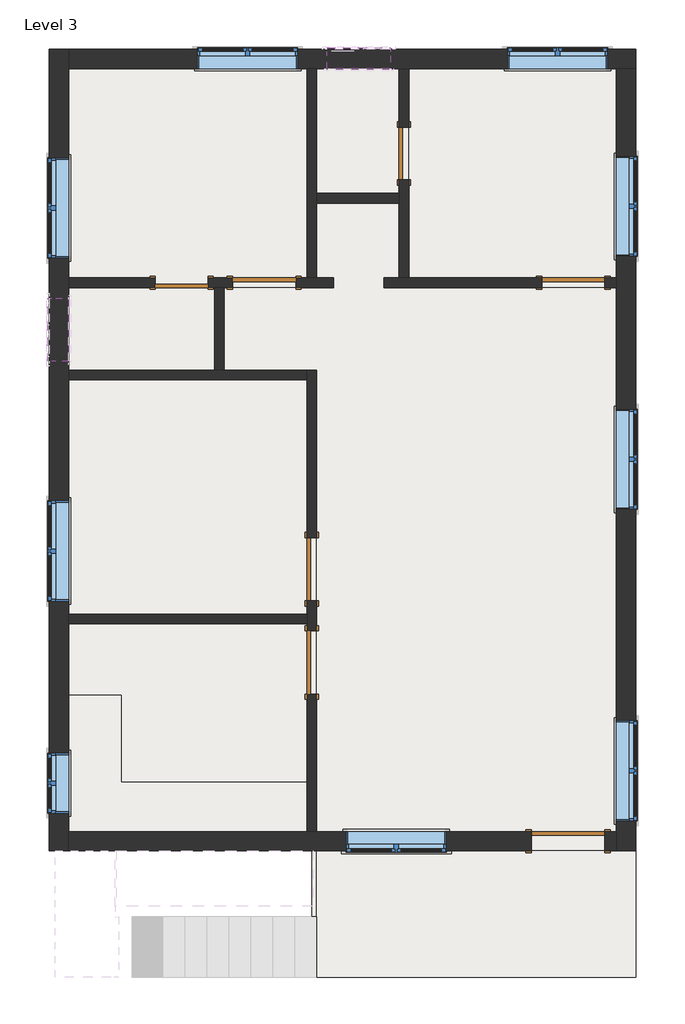
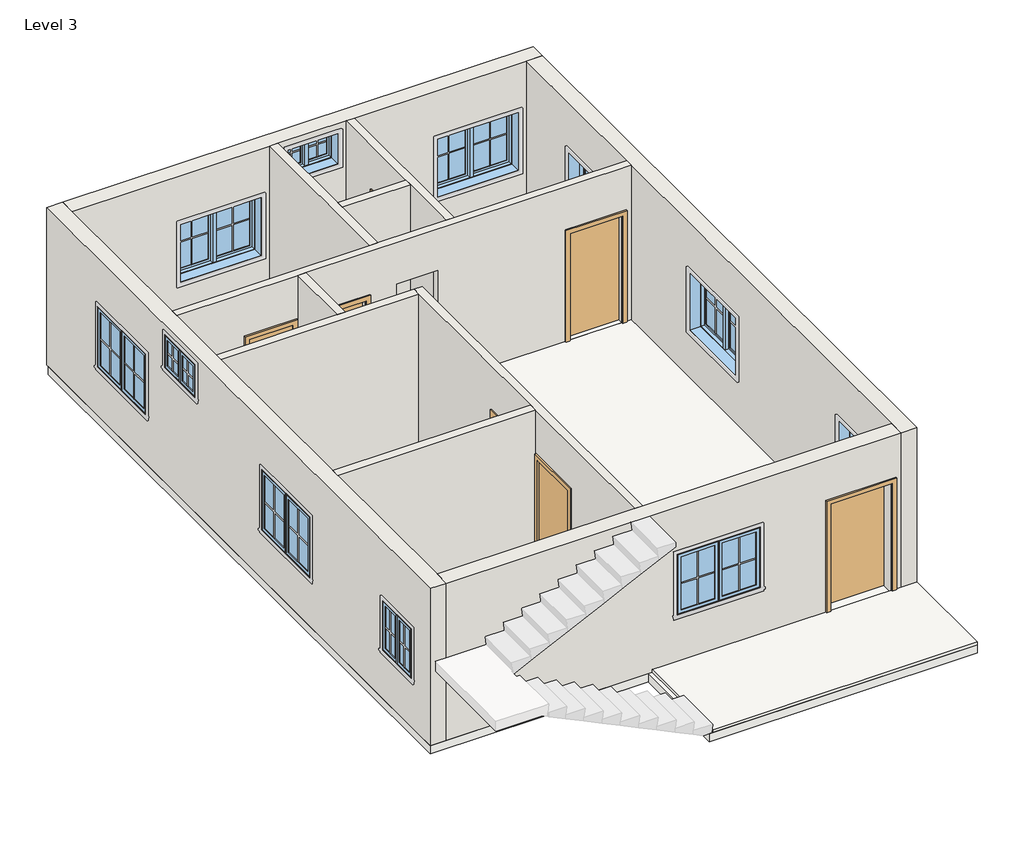
# One storey, part 1 of 2: 12 walls, 11 windows, 7 doors, 6 slabs.
"""IFC4 building model written with IfcOpenShell, lengths in millimetres."""

from ifc_helpers import new_model, si_unit, frame, origin, place, context, project, spatial, polyline, outline, extrude, faceted_brep, transform, mapped, element, save
from components import single_flush_3_6_472124c4, door_c78455d5, door_ad1ac78c, door_798417c2, window_casement_double_3_v2_9f1923e6, window_6eb120d7, window_2333f571

model = new_model("IFC4")

# Units and contexts
model_context = context("Model", 3, world=origin())
ifc_project = project(units=[si_unit("LENGTHUNIT", "METRE", prefix="MILLI")], contexts=[model_context])

# Site, building, storey
site = spatial("IfcSite", under=ifc_project)
building = spatial("IfcBuilding", under=site)
storey = spatial("IfcBuildingStorey", under=building, Name="Level 3", Elevation=6096.0)

# Doors
placement = place(None, origin())
single_flush_3_6_shape = single_flush_3_6_472124c4(model_context)
element("IfcDoor", 1, ObjectType="Single-Flush : 3'6", at=placement, inside=storey, context=model_context, shape_type="MappedRepresentation", body=[
    mapped(single_flush_3_6_shape, transform((-1353.6785282, -4927.3203663, 6096.0), x_axis=(1.0, 0.0, 0.0), y_axis=(0.0, 1.0, 0.0), z_axis=(0.0, 0.0, 1.0))),
])
door_shape = door_c78455d5(model_context)
element("IfcDoor", 2, ObjectType="Single-Flush : 30\" x 80\"", at=placement, inside=storey, context=model_context, shape_type="MappedRepresentation", body=[
    mapped(door_shape, transform((-6936.6570389, 3131.9303819, 6096.0), x_axis=(1.0, 0.0, 0.0), y_axis=(0.0, 1.0, 0.0), z_axis=(0.0, 0.0, 1.0))),
])
element("IfcDoor", 3, ObjectType="Single-Flush : 30\" x 80\"", at=placement, inside=storey, context=model_context, shape_type="MappedRepresentation", body=[
    mapped(door_shape, transform((-3724.1740631, 4999.2141951, 6096.0), x_axis=(0.0, -1.0, 0.0), y_axis=(1.0, 0.0, 0.0), z_axis=(0.0, 0.0, 1.0))),
])
door_2_shape = door_ad1ac78c(model_context)
element("IfcDoor", 4, ObjectType="Single-Flush : 36\" x 80\"", at=placement, inside=storey, context=model_context, shape_type="MappedRepresentation", body=[
    mapped(door_2_shape, transform((-5742.8570389, 3131.9303819, 6096.0), x_axis=(1.0, 0.0, 0.0), y_axis=(0.0, 1.0, 0.0), z_axis=(0.0, 0.0, 1.0))),
])
element("IfcDoor", 5, ObjectType="Single-Flush : 36\" x 80\"", at=placement, inside=storey, context=model_context, shape_type="MappedRepresentation", body=[
    mapped(door_2_shape, transform((-1277.4785282, 3131.9303819, 6096.0), x_axis=(1.0, 0.0, 0.0), y_axis=(0.0, 1.0, 0.0), z_axis=(0.0, 0.0, 1.0))),
])
element("IfcDoor", 6, ObjectType="Single-Flush : 36\" x 80\"", at=placement, inside=storey, context=model_context, shape_type="MappedRepresentation", body=[
    mapped(door_2_shape, transform((-5055.0449828, -2348.5368209, 6096.0), x_axis=(0.0, 1.0, 0.0), y_axis=(-1.0, 0.0, 0.0), z_axis=(0.0, 0.0, 1.0))),
])
door_3_shape = door_798417c2(model_context)
element("IfcDoor", 7, ObjectType="Single-Flush : 36\" x 80\"", at=placement, inside=storey, context=model_context, shape_type="MappedRepresentation", body=[
    mapped(door_3_shape, transform((-5055.0449828, -1002.3368209, 6096.0), x_axis=(0.0, -1.0, 0.0), y_axis=(1.0, 0.0, 0.0), z_axis=(0.0, 0.0, 1.0))),
])

# Slabs
element("IfcSlab", 8, ObjectType="6\"", at=placement, inside=storey, context=model_context, shape_type="SweptSolid", body=[
    extrude(outline(polyline([(-375.7785282, 6451.8796337), (-375.7785282, -6894.0922127), (-5049.0296925, -6894.0922127), (-5049.0296925, -5067.0203663), (-8849.1884077, -5067.0203663), (-8849.1884077, 6451.8796337), (-375.7785282, 6451.8796337)])), frame((0.0, 0.0, 5943.6), z_axis=(0.0, 0.0, 1.0), x_axis=(1.0, 0.0, 0.0)), (0.0, 0.0, 1.0), 152.4),
])
element("IfcSlab", 9, ObjectType="BED ROOM FLOOR", at=placement, inside=storey, context=model_context, shape_type="SweptSolid", body=[
    extrude(outline(polyline([(-4985.1949828, -4787.6203663), (-8569.7884077, -4787.6203663), (-8569.7884077, -1788.4748314), (-4985.1949828, -1788.4748314), (-4985.1949828, -4787.6203663)])), frame((0.0, 0.0, 6096.0), z_axis=(0.0, 0.0, 1.0), x_axis=(1.0, 0.0, 0.0)), (0.0, 0.0, 1.0), 50.8),
    extrude(outline(polyline([(-4985.1949828, -1672.5465885), (-8569.7884077, -1672.5465885), (-8569.7884077, 1731.1760727), (-4985.1949828, 1731.1760727), (-4985.1949828, -1672.5465885)])), frame((0.0, 0.0, 6096.0), z_axis=(0.0, 0.0, 1.0), x_axis=(1.0, 0.0, 0.0)), (0.0, 0.0, 1.0), 50.8),
    extrude(outline(polyline([(-8569.7884077, 6224.6642844), (-5124.8949828, 6224.6642844), (-5124.8949828, 3062.0803819), (-8569.7884077, 3062.0803819), (-8569.7884077, 6224.6642844)])), frame((0.0, 0.0, 6096.0), z_axis=(0.0, 0.0, 1.0), x_axis=(1.0, 0.0, 0.0)), (0.0, 0.0, 1.0), 50.8),
    extrude(outline(polyline([(-655.1785282, 6224.6642844), (-655.1785282, 3062.0803819), (-3654.3240631, 3062.0803819), (-3654.3240631, 6224.6642844), (-655.1785282, 6224.6642844)])), frame((0.0, 0.0, 6096.0), z_axis=(0.0, 0.0, 1.0), x_axis=(1.0, 0.0, 0.0)), (0.0, 0.0, 1.0), 50.8),
])
element("IfcSlab", 10, ObjectType="HALL FLOOR", at=placement, inside=storey, context=model_context, shape_type="SweptSolid", body=[
    extrude(outline(polyline([(-4985.1949828, -4787.6203663), (-4985.1949828, 1842.4631791), (-6320.7070389, 1842.4631791), (-6320.7070389, 3062.0803819), (-4744.7849815, 3062.0803819), (-4744.7849815, 3178.0086247), (-4985.1949828, 3178.0086247), (-4985.1949828, 4281.6641951), (-3765.6111695, 4281.6641951), (-3765.6111695, 3178.0086247), (-3997.4676553, 3178.0086247), (-3997.4676553, 3062.0803819), (-655.1785282, 3062.0803819), (-655.1785282, -4787.6203663), (-4985.1949828, -4787.6203663)])), frame((0.0, 0.0, 6096.0), z_axis=(0.0, 0.0, 1.0), x_axis=(1.0, 0.0, 0.0)), (0.0, 0.0, 1.0), 50.8),
])
element("IfcSlab", 11, ObjectType="HALL FLOOR", at=placement, inside=storey, context=model_context, shape_type="SweptSolid", body=[
    extrude(outline(polyline([(-375.7785282, -5067.0203663), (-375.7785282, -6894.0922127), (-4985.1949828, -6894.0922127), (-4985.1949828, -5067.0203663), (-375.7785282, -5067.0203663)])), frame((0.0, 0.0, 6096.0), z_axis=(0.0, 0.0, 1.0), x_axis=(1.0, 0.0, 0.0)), (0.0, 0.0, 1.0), 50.8),
])
element("IfcSlab", 12, ObjectType="KITCHEN BED", at=placement, inside=storey, context=model_context, shape_type="SweptSolid", body=[
    extrude(outline(polyline([(-7807.7884077, -2823.0618171), (-7807.7884077, -4077.7716275), (-5124.8949828, -4077.7716275), (-5124.8949828, -4839.7716275), (-7807.7884077, -4839.7716275), (-8569.7884077, -4839.7716275), (-8569.7884077, -2823.0618171), (-7807.7884077, -2823.0618171)])), frame((0.0, 0.0, 6908.8), z_axis=(0.0, 0.0, 1.0), x_axis=(1.0, 0.0, 0.0)), (0.0, 0.0, 1.0), 101.6),
])
element("IfcSlab", 13, ObjectType="TOILET FLOORING", at=placement, inside=storey, context=model_context, shape_type="SweptSolid", body=[
    extrude(outline(polyline([(-6432.0275348, 3201.7803819), (-6432.0275348, 1842.4631791), (-8569.7884077, 1842.4631791), (-8569.7884077, 3201.7803819), (-6432.0275348, 3201.7803819)])), frame((0.0, 0.0, 6096.0), z_axis=(0.0, 0.0, 1.0), x_axis=(1.0, 0.0, 0.0)), (0.0, 0.0, 1.0), 50.8),
    extrude(outline(polyline([(-3654.3240631, 6224.6642844), (-3654.3240631, 4397.592438), (-4985.1949828, 4397.592438), (-4985.1949828, 6224.6642844), (-3654.3240631, 6224.6642844)])), frame((0.0, 0.0, 6096.0), z_axis=(0.0, 0.0, 1.0), x_axis=(1.0, 0.0, 0.0)), (0.0, 0.0, 1.0), 50.8),
])

# Walls
element("IfcWall", 14, ObjectType="4.5\"", at=placement, inside=storey, context=model_context, shape_type="Brep", body=[
    faceted_brep([(-5124.8949828, -1459.5368209, 6096.0), (-5124.8949828, -1648.7748314, 6096.0), (-5124.8949828, -1788.4748314, 6096.0), (-5124.8949828, -1891.3368209, 6096.0), (-5124.8949828, -1891.3368209, 8128.0), (-5124.8949828, -2805.7368209, 8128.0), (-5124.8949828, -2805.7368209, 6096.0), (-5124.8949828, -4787.6203663, 6096.0), (-5124.8949828, -4787.6203663, 8991.6), (-5124.8949828, -1788.4748314, 8991.6), (-5124.8949828, -1648.7748314, 8991.6), (-5124.8949828, 1731.1760727, 8991.6), (-5124.8949828, 1870.8760727, 8991.6), (-5124.8949828, 1870.8760727, 6096.0), (-5124.8949828, 1731.1760727, 6096.0), (-5124.8949828, -545.1368209, 6096.0), (-5124.8949828, -545.1368209, 8128.0), (-5124.8949828, -1459.5368209, 8128.0), (-4985.1949828, -1891.3368209, 8128.0), (-4985.1949828, -1891.3368209, 6096.0), (-4985.1949828, -1459.5368209, 6096.0), (-4985.1949828, -1459.5368209, 8128.0), (-4985.1949828, -545.1368209, 8128.0), (-4985.1949828, -545.1368209, 6096.0), (-4985.1949828, 1870.8760727, 6096.0), (-4985.1949828, 1870.8760727, 8991.6), (-4985.1949828, -4787.6203663, 8991.6), (-4985.1949828, -4787.6203663, 6096.0), (-4985.1949828, -2805.7368209, 6096.0), (-4985.1949828, -2805.7368209, 8128.0)], [[[0, 1, 2, 3, 4, 5, 6, 7, 8, 9, 10, 11, 12, 13, 14, 15, 16, 17]], [[18, 19, 20, 21, 22, 23, 24, 25, 26, 27, 28, 29]], [[28, 27, 7, 6]], [[20, 19, 3, 2, 1, 0]], [[15, 14, 13, 24, 23]], [[12, 11, 10, 9, 8, 26, 25]], [[8, 7, 27, 26]], [[21, 20, 0, 17]], [[22, 21, 17, 16]], [[23, 22, 16, 15]], [[4, 3, 19, 18]], [[5, 4, 18, 29]], [[6, 5, 29, 28]], [[13, 12, 25, 24]]]),
])
element("IfcWall", 15, ObjectType="4.5\"", at=placement, inside=storey, context=model_context, shape_type="SweptSolid", body=[
    extrude(outline(polyline([(-8569.7884077, -1648.7748314), (-5124.8949828, -1648.7748314), (-5124.8949828, -1788.4748314), (-8569.7884077, -1788.4748314), (-8569.7884077, -1648.7748314)])), frame((0.0, 0.0, 6096.0), z_axis=(0.0, 0.0, 1.0), x_axis=(1.0, 0.0, 0.0)), (0.0, 0.0, 1.0), 2895.6),
])
element("IfcWall", 16, ObjectType="4.5\"", at=placement, inside=storey, context=model_context, shape_type="Brep", body=[
    faceted_brep([(-5124.8949828, 1870.8760727, 6096.0), (-6320.7070389, 1870.8760727, 6096.0), (-6460.4070389, 1870.8760727, 6096.0), (-8569.7884077, 1870.8760727, 6096.0), (-8569.7884077, 1870.8760727, 8991.6), (-6460.4070389, 1870.8760727, 8991.6), (-6320.7070389, 1870.8760727, 8991.6), (-5124.8949828, 1870.8760727, 8991.6), (-5124.8949828, 1731.1760727, 6096.0), (-5124.8949828, 1731.1760727, 8991.6), (-8569.7884077, 1731.1760727, 8991.6), (-8569.7884077, 1731.1760727, 6096.0)], [[[0, 1, 2, 3, 4, 5, 6, 7]], [[8, 9, 10, 11]], [[3, 2, 1, 0, 8, 11]], [[7, 6, 5, 4, 10, 9]], [[4, 3, 11, 10]], [[0, 7, 9, 8]]]),
])
element("IfcWall", 17, ObjectType="4.5\"", at=placement, inside=storey, context=model_context, shape_type="SweptSolid", body=[
    extrude(outline(polyline([(-6460.4070389, 1870.8760727), (-6460.4070389, 3062.0803819), (-6320.7070389, 3062.0803819), (-6320.7070389, 1870.8760727), (-6460.4070389, 1870.8760727)])), frame((0.0, 0.0, 6096.0), z_axis=(0.0, 0.0, 1.0), x_axis=(1.0, 0.0, 0.0)), (0.0, 0.0, 1.0), 2895.6),
])
element("IfcWall", 18, ObjectType="4.5\"", at=placement, inside=storey, context=model_context, shape_type="Brep", body=[
    faceted_brep([(-6200.0570389, 3201.7803819, 6096.0), (-6555.6570389, 3201.7803819, 6096.0), (-6555.6570389, 3201.7803819, 8128.0), (-7317.6570389, 3201.7803819, 8128.0), (-7317.6570389, 3201.7803819, 6096.0), (-8569.7884077, 3201.7803819, 6096.0), (-8569.7884077, 3201.7803819, 8991.6), (-5124.8949828, 3201.7803819, 8991.6), (-4985.1949828, 3201.7803819, 8991.6), (-3794.0240631, 3201.7803819, 8991.6), (-3654.3240631, 3201.7803819, 8991.6), (-655.1785282, 3201.7803819, 8991.6), (-655.1785282, 3201.7803819, 6096.0), (-820.2785282, 3201.7803819, 6096.0), (-820.2785282, 3201.7803819, 8128.0), (-1734.6785282, 3201.7803819, 8128.0), (-1734.6785282, 3201.7803819, 6096.0), (-3654.3240631, 3201.7803819, 6096.0), (-3794.0240631, 3201.7803819, 6096.0), (-4012.6375241, 3201.7803819, 6096.0), (-4012.6375241, 3201.7803819, 8229.6), (-4744.7849815, 3201.7803819, 8229.6), (-4744.7849815, 3201.7803819, 6096.0), (-4985.1949828, 3201.7803819, 6096.0), (-5124.8949828, 3201.7803819, 6096.0), (-5285.6570389, 3201.7803819, 6096.0), (-5285.6570389, 3201.7803819, 8128.0), (-6200.0570389, 3201.7803819, 8128.0), (-6555.6570389, 3062.0803819, 8128.0), (-6555.6570389, 3062.0803819, 6096.0), (-6460.4070389, 3062.0803819, 6096.0), (-6320.7070389, 3062.0803819, 6096.0), (-6200.0570389, 3062.0803819, 6096.0), (-6200.0570389, 3062.0803819, 8128.0), (-5285.6570389, 3062.0803819, 8128.0), (-5285.6570389, 3062.0803819, 6096.0), (-4744.7849815, 3062.0803819, 6096.0), (-4744.7849815, 3062.0803819, 8229.6), (-4012.6375241, 3062.0803819, 8229.6), (-4012.6375241, 3062.0803819, 6096.0), (-1734.6785282, 3062.0803819, 6096.0), (-1734.6785282, 3062.0803819, 8128.0), (-820.2785282, 3062.0803819, 8128.0), (-820.2785282, 3062.0803819, 6096.0), (-655.1785282, 3062.0803819, 6096.0), (-655.1785282, 3062.0803819, 8991.6), (-6320.7070389, 3062.0803819, 8991.6), (-6460.4070389, 3062.0803819, 8991.6), (-8569.7884077, 3062.0803819, 8991.6), (-8569.7884077, 3062.0803819, 6096.0), (-7317.6570389, 3062.0803819, 6096.0), (-7317.6570389, 3062.0803819, 8128.0)], [[[0, 1, 2, 3, 4, 5, 6, 7, 8, 9, 10, 11, 12, 13, 14, 15, 16, 17, 18, 19, 20, 21, 22, 23, 24, 25, 26, 27]], [[28, 29, 30, 31, 32, 33, 34, 35, 36, 37, 38, 39, 40, 41, 42, 43, 44, 45, 46, 47, 48, 49, 50, 51]], [[36, 35, 25, 24, 23, 22]], [[40, 39, 19, 18, 17, 16]], [[44, 43, 13, 12]], [[50, 49, 5, 4]], [[32, 31, 30, 29, 1, 0]], [[11, 10, 9, 8, 7, 6, 48, 47, 46, 45]], [[6, 5, 49, 48]], [[12, 11, 45, 44]], [[20, 38, 37, 21]], [[38, 20, 19, 39]], [[21, 37, 36, 22]], [[26, 25, 35, 34]], [[27, 26, 34, 33]], [[0, 27, 33, 32]], [[14, 13, 43, 42]], [[15, 14, 42, 41]], [[16, 15, 41, 40]], [[2, 1, 29, 28]], [[3, 2, 28, 51]], [[4, 3, 51, 50]]]),
])
element("IfcWall", 19, ObjectType="4.5\"", at=placement, inside=storey, context=model_context, shape_type="Brep", body=[
    faceted_brep([(-5124.8949828, 6224.6642844, 6096.0), (-5124.8949828, 3201.7803819, 6096.0), (-5124.8949828, 3201.7803819, 8991.6), (-5124.8949828, 6224.6642844, 8991.6), (-4985.1949828, 6224.6642844, 6096.0), (-4985.1949828, 6224.6642844, 8991.6), (-4985.1949828, 4421.3641951, 8991.6), (-4985.1949828, 4281.6641951, 8991.6), (-4985.1949828, 3201.7803819, 8991.6), (-4985.1949828, 3201.7803819, 6096.0), (-4985.1949828, 4281.6641951, 6096.0), (-4985.1949828, 4421.3641951, 6096.0)], [[[0, 1, 2, 3]], [[4, 5, 6, 7, 8, 9, 10, 11]], [[1, 0, 4, 11, 10, 9]], [[3, 2, 8, 7, 6, 5]], [[0, 3, 5, 4]], [[2, 1, 9, 8]]]),
])
element("IfcWall", 20, ObjectType="4.5\"", at=placement, inside=storey, context=model_context, shape_type="Brep", body=[
    faceted_brep([(-3794.0240631, 4618.2141951, 8128.0), (-3794.0240631, 4618.2141951, 6096.0), (-3794.0240631, 4421.3641951, 6096.0), (-3794.0240631, 4281.6641951, 6096.0), (-3794.0240631, 3201.7803819, 6096.0), (-3794.0240631, 3201.7803819, 8991.6), (-3794.0240631, 4281.6641951, 8991.6), (-3794.0240631, 4421.3641951, 8991.6), (-3794.0240631, 6224.6642844, 8991.6), (-3794.0240631, 6224.6642844, 6096.0), (-3794.0240631, 5380.2141951, 6096.0), (-3794.0240631, 5380.2141951, 8128.0), (-3654.3240631, 3201.7803819, 6096.0), (-3654.3240631, 4618.2141951, 6096.0), (-3654.3240631, 4618.2141951, 8128.0), (-3654.3240631, 5380.2141951, 8128.0), (-3654.3240631, 5380.2141951, 6096.0), (-3654.3240631, 6224.6642844, 6096.0), (-3654.3240631, 6224.6642844, 8991.6), (-3654.3240631, 3201.7803819, 8991.6)], [[[0, 1, 2, 3, 4, 5, 6, 7, 8, 9, 10, 11]], [[12, 13, 14, 15, 16, 17, 18, 19]], [[10, 9, 17, 16]], [[4, 3, 2, 1, 13, 12]], [[8, 7, 6, 5, 19, 18]], [[9, 8, 18, 17]], [[14, 13, 1, 0]], [[15, 14, 0, 11]], [[16, 15, 11, 10]], [[5, 4, 12, 19]]]),
])
element("IfcWall", 21, ObjectType="4.5\"", at=placement, inside=storey, context=model_context, shape_type="SweptSolid", body=[
    extrude(outline(polyline([(-4985.1949828, 4421.3641951), (-3794.0240631, 4421.3641951), (-3794.0240631, 4281.6641951), (-4985.1949828, 4281.6641951), (-4985.1949828, 4421.3641951)])), frame((0.0, 0.0, 6096.0), z_axis=(0.0, 0.0, 1.0), x_axis=(1.0, 0.0, 0.0)), (0.0, 0.0, 1.0), 2895.6),
])
element("IfcWall", 22, ObjectType="9\"", at=placement, inside=storey, context=model_context, shape_type="Brep", body=[
    faceted_brep([(-8849.1884077, 6504.0642844, 6096.0), (-8849.1884077, -5067.0203663, 6096.0), (-8849.1884077, -5067.0203663, 8991.6), (-8849.1884077, 6504.0642844, 8991.6), (-8849.1884077, -3657.3203663, 7924.8), (-8849.1884077, -4520.9203663, 7924.8), (-8849.1884077, -4520.9203663, 7010.4), (-8849.1884077, -3657.3203663, 7010.4), (-8849.1884077, 4935.3303819, 8128.0), (-8849.1884077, 3487.5303819, 8128.0), (-8849.1884077, 3487.5303819, 7010.4), (-8849.1884077, 4935.3303819, 7010.4), (-8849.1884077, -16.8248314, 8128.0), (-8849.1884077, -1464.6248314, 8128.0), (-8849.1884077, -1464.6248314, 7010.4), (-8849.1884077, -16.8248314, 7010.4), (-8849.1884077, 2910.9782273, 8839.2), (-8849.1884077, 1996.5782273, 8839.2), (-8849.1884077, 1996.5782273, 8229.6), (-8849.1884077, 2910.9782273, 8229.6), (-8569.7884077, 6504.0642844, 6096.0), (-8569.7884077, 6504.0642844, 8991.6), (-8569.7884077, 6224.6642844, 8991.6), (-8569.7884077, 3201.7803819, 8991.6), (-8569.7884077, 3062.0803819, 8991.6), (-8569.7884077, 1870.8760727, 8991.6), (-8569.7884077, 1731.1760727, 8991.6), (-8569.7884077, -1648.7748314, 8991.6), (-8569.7884077, -1788.4748314, 8991.6), (-8569.7884077, -4787.6203663, 8991.6), (-8569.7884077, -5067.0203663, 8991.6), (-8569.7884077, -5067.0203663, 6096.0), (-8569.7884077, -4787.6203663, 6096.0), (-8569.7884077, -1788.4748314, 6096.0), (-8569.7884077, -1648.7748314, 6096.0), (-8569.7884077, 1731.1760727, 6096.0), (-8569.7884077, 1870.8760727, 6096.0), (-8569.7884077, 3062.0803819, 6096.0), (-8569.7884077, 3201.7803819, 6096.0), (-8569.7884077, 6224.6642844, 6096.0), (-8569.7884077, -3657.3203663, 7924.8), (-8569.7884077, -3657.3203663, 7010.4), (-8569.7884077, -4520.9203663, 7010.4), (-8569.7884077, -4520.9203663, 7924.8), (-8569.7884077, 4935.3303819, 8128.0), (-8569.7884077, 4935.3303819, 7010.4), (-8569.7884077, 3487.5303819, 7010.4), (-8569.7884077, 3487.5303819, 8128.0), (-8569.7884077, -16.8248314, 8128.0), (-8569.7884077, -16.8248314, 7010.4), (-8569.7884077, -1464.6248314, 7010.4), (-8569.7884077, -1464.6248314, 8128.0), (-8569.7884077, 2910.9782273, 8839.2), (-8569.7884077, 2910.9782273, 8229.6), (-8569.7884077, 1996.5782273, 8229.6), (-8569.7884077, 1996.5782273, 8839.2)], [[[0, 1, 2, 3], [4, 5, 6, 7], [8, 9, 10, 11], [12, 13, 14, 15], [16, 17, 18, 19]], [[20, 21, 22, 23, 24, 25, 26, 27, 28, 29, 30, 31, 32, 33, 34, 35, 36, 37, 38, 39], [40, 41, 42, 43], [44, 45, 46, 47], [48, 49, 50, 51], [52, 53, 54, 55]], [[1, 0, 20, 39, 38, 37, 36, 35, 34, 33, 32, 31]], [[3, 2, 30, 29, 28, 27, 26, 25, 24, 23, 22, 21]], [[0, 3, 21, 20]], [[2, 1, 31, 30]], [[41, 40, 4, 7]], [[42, 41, 7, 6]], [[43, 42, 6, 5]], [[40, 43, 5, 4]], [[45, 44, 8, 11]], [[46, 45, 11, 10]], [[47, 46, 10, 9]], [[44, 47, 9, 8]], [[49, 48, 12, 15]], [[50, 49, 15, 14]], [[51, 50, 14, 13]], [[48, 51, 13, 12]], [[53, 52, 16, 19]], [[54, 53, 19, 18]], [[55, 54, 18, 17]], [[52, 55, 17, 16]]]),
])
element("IfcWall", 23, ObjectType="9\"", at=placement, inside=storey, context=model_context, shape_type="Brep", body=[
    faceted_brep([(-375.7785282, 6504.0642844, 6096.0), (-8569.7884077, 6504.0642844, 6096.0), (-8569.7884077, 6504.0642844, 8991.6), (-375.7785282, 6504.0642844, 8991.6), (-782.1785282, 6504.0642844, 8128.0), (-2229.9785282, 6504.0642844, 8128.0), (-2229.9785282, 6504.0642844, 7010.4), (-782.1785282, 6504.0642844, 7010.4), (-5258.2449828, 6504.0642844, 8128.0), (-6706.0449828, 6504.0642844, 8128.0), (-6706.0449828, 6504.0642844, 7010.4), (-5258.2449828, 6504.0642844, 7010.4), (-3919.7095229, 6504.0642844, 8839.2), (-4834.1095229, 6504.0642844, 8839.2), (-4834.1095229, 6504.0642844, 8229.6), (-3919.7095229, 6504.0642844, 8229.6), (-375.7785282, 6224.6642844, 6096.0), (-375.7785282, 6224.6642844, 8991.6), (-655.1785282, 6224.6642844, 8991.6), (-3654.3240631, 6224.6642844, 8991.6), (-3794.0240631, 6224.6642844, 8991.6), (-4985.1949828, 6224.6642844, 8991.6), (-5124.8949828, 6224.6642844, 8991.6), (-8569.7884077, 6224.6642844, 8991.6), (-8569.7884077, 6224.6642844, 6096.0), (-5124.8949828, 6224.6642844, 6096.0), (-4985.1949828, 6224.6642844, 6096.0), (-3794.0240631, 6224.6642844, 6096.0), (-3654.3240631, 6224.6642844, 6096.0), (-655.1785282, 6224.6642844, 6096.0), (-782.1785282, 6224.6642844, 8128.0), (-782.1785282, 6224.6642844, 7010.4), (-2229.9785282, 6224.6642844, 7010.4), (-2229.9785282, 6224.6642844, 8128.0), (-5258.2449828, 6224.6642844, 8128.0), (-5258.2449828, 6224.6642844, 7010.4), (-6706.0449828, 6224.6642844, 7010.4), (-6706.0449828, 6224.6642844, 8128.0), (-3919.7095229, 6224.6642844, 8839.2), (-3919.7095229, 6224.6642844, 8229.6), (-4834.1095229, 6224.6642844, 8229.6), (-4834.1095229, 6224.6642844, 8839.2)], [[[0, 1, 2, 3], [4, 5, 6, 7], [8, 9, 10, 11], [12, 13, 14, 15]], [[16, 17, 18, 19, 20, 21, 22, 23, 24, 25, 26, 27, 28, 29], [30, 31, 32, 33], [34, 35, 36, 37], [38, 39, 40, 41]], [[1, 0, 16, 29, 28, 27, 26, 25, 24]], [[3, 2, 23, 22, 21, 20, 19, 18, 17]], [[2, 1, 24, 23]], [[0, 3, 17, 16]], [[31, 30, 4, 7]], [[32, 31, 7, 6]], [[33, 32, 6, 5]], [[30, 33, 5, 4]], [[35, 34, 8, 11]], [[36, 35, 11, 10]], [[37, 36, 10, 9]], [[34, 37, 9, 8]], [[39, 38, 12, 15]], [[40, 39, 15, 14]], [[41, 40, 14, 13]], [[38, 41, 13, 12]]]),
])
element("IfcWall", 24, ObjectType="9\"", at=placement, inside=storey, context=model_context, shape_type="Brep", body=[
    faceted_brep([(-655.1785282, 6224.6642844, 6096.0), (-655.1785282, 3201.7803819, 6096.0), (-655.1785282, 3062.0803819, 6096.0), (-655.1785282, -4787.6203663, 6096.0), (-655.1785282, -5067.0203663, 6096.0), (-655.1785282, -5067.0203663, 8991.6), (-655.1785282, -4787.6203663, 8991.6), (-655.1785282, 3062.0803819, 8991.6), (-655.1785282, 3201.7803819, 8991.6), (-655.1785282, 6224.6642844, 8991.6), (-655.1785282, -4635.2203663, 8128.0), (-655.1785282, -4635.2203663, 7010.4), (-655.1785282, -3187.4203663, 7010.4), (-655.1785282, -3187.4203663, 8128.0), (-655.1785282, -139.4203663, 8128.0), (-655.1785282, -139.4203663, 7010.4), (-655.1785282, 1308.3796337, 7010.4), (-655.1785282, 1308.3796337, 8128.0), (-655.1785282, 3512.9303819, 8128.0), (-655.1785282, 3512.9303819, 7010.4), (-655.1785282, 4960.7303819, 7010.4), (-655.1785282, 4960.7303819, 8128.0), (-375.7785282, 6224.6642844, 6096.0), (-375.7785282, 6224.6642844, 8991.6), (-375.7785282, -5067.0203663, 8991.6), (-375.7785282, -5067.0203663, 6096.0), (-375.7785282, -4635.2203663, 8128.0), (-375.7785282, -3187.4203663, 8128.0), (-375.7785282, -3187.4203663, 7010.4), (-375.7785282, -4635.2203663, 7010.4), (-375.7785282, -139.4203663, 8128.0), (-375.7785282, 1308.3796337, 8128.0), (-375.7785282, 1308.3796337, 7010.4), (-375.7785282, -139.4203663, 7010.4), (-375.7785282, 3512.9303819, 8128.0), (-375.7785282, 4960.7303819, 8128.0), (-375.7785282, 4960.7303819, 7010.4), (-375.7785282, 3512.9303819, 7010.4)], [[[0, 1, 2, 3, 4, 5, 6, 7, 8, 9], [10, 11, 12, 13], [14, 15, 16, 17], [18, 19, 20, 21]], [[22, 23, 24, 25], [26, 27, 28, 29], [30, 31, 32, 33], [34, 35, 36, 37]], [[4, 3, 2, 1, 0, 22, 25]], [[9, 8, 7, 6, 5, 24, 23]], [[5, 4, 25, 24]], [[0, 9, 23, 22]], [[11, 10, 26, 29]], [[12, 11, 29, 28]], [[13, 12, 28, 27]], [[10, 13, 27, 26]], [[15, 14, 30, 33]], [[16, 15, 33, 32]], [[17, 16, 32, 31]], [[14, 17, 31, 30]], [[19, 18, 34, 37]], [[20, 19, 37, 36]], [[21, 20, 36, 35]], [[18, 21, 35, 34]]]),
])
element("IfcWall", 25, ObjectType="9\"", at=placement, inside=storey, context=model_context, shape_type="Brep", body=[
    faceted_brep([(-655.1785282, -4787.6203663, 6096.0), (-820.2785282, -4787.6203663, 6096.0), (-820.2785282, -4787.6203663, 8128.0), (-1887.0785282, -4787.6203663, 8128.0), (-1887.0785282, -4787.6203663, 6096.0), (-4985.1949828, -4787.6203663, 6096.0), (-5124.8949828, -4787.6203663, 6096.0), (-8569.7884077, -4787.6203663, 6096.0), (-8569.7884077, -4787.6203663, 8991.6), (-5124.8949828, -4787.6203663, 8991.6), (-4985.1949828, -4787.6203663, 8991.6), (-655.1785282, -4787.6203663, 8991.6), (-4559.7449828, -4787.6203663, 8128.0), (-4559.7449828, -4787.6203663, 7010.4), (-3111.9449828, -4787.6203663, 7010.4), (-3111.9449828, -4787.6203663, 8128.0), (-820.2785282, -5067.0203663, 8128.0), (-820.2785282, -5067.0203663, 6096.0), (-655.1785282, -5067.0203663, 6096.0), (-655.1785282, -5067.0203663, 8991.6), (-8569.7884077, -5067.0203663, 8991.6), (-8569.7884077, -5067.0203663, 6096.0), (-1887.0785282, -5067.0203663, 6096.0), (-1887.0785282, -5067.0203663, 8128.0), (-4559.7449828, -5067.0203663, 8128.0), (-3111.9449828, -5067.0203663, 8128.0), (-3111.9449828, -5067.0203663, 7010.4), (-4559.7449828, -5067.0203663, 7010.4)], [[[0, 1, 2, 3, 4, 5, 6, 7, 8, 9, 10, 11], [12, 13, 14, 15]], [[16, 17, 18, 19, 20, 21, 22, 23], [24, 25, 26, 27]], [[22, 21, 7, 6, 5, 4]], [[18, 17, 1, 0]], [[11, 10, 9, 8, 20, 19]], [[0, 11, 19, 18]], [[8, 7, 21, 20]], [[13, 12, 24, 27]], [[14, 13, 27, 26]], [[15, 14, 26, 25]], [[12, 15, 25, 24]], [[2, 1, 17, 16]], [[3, 2, 16, 23]], [[4, 3, 23, 22]]]),
])

# Windows
window_casement_double_3_v2_shape = window_casement_double_3_v2_9f1923e6(model_context)
element("IfcWindow", 26, ObjectType="Window-Casement-Double : 3'V2'", at=placement, inside=storey, context=model_context, shape_type="MappedRepresentation", body=[
    mapped(window_casement_double_3_v2_shape, transform((-8709.4884077, 2453.7782273, 7315.2), x_axis=(0.0, 1.0, 0.0), y_axis=(-1.0, 0.0, 0.0), z_axis=(0.0, 0.0, 1.0))),
])
element("IfcWindow", 27, ObjectType="Window-Casement-Double : 3'V2'", at=placement, inside=storey, context=model_context, shape_type="MappedRepresentation", body=[
    mapped(window_casement_double_3_v2_shape, transform((-4376.9095229, 6364.3642844, 7315.2), x_axis=(1.0, 0.0, 0.0), y_axis=(0.0, 1.0, 0.0), z_axis=(0.0, 0.0, 1.0))),
])
window_shape = window_6eb120d7(model_context)
element("IfcWindow", 28, ObjectType="Window-Casement-Double : 34\" x 36\"", at=placement, inside=storey, context=model_context, shape_type="MappedRepresentation", body=[
    mapped(window_shape, transform((-8709.4884077, -4089.1203663, 6096.0), x_axis=(0.0, 1.0, 0.0), y_axis=(-1.0, 0.0, 0.0), z_axis=(0.0, 0.0, 1.0))),
])
window_2_shape = window_2333f571(model_context)
element("IfcWindow", 29, ObjectType="Window-Casement-Double : 57\" x 44\"", at=placement, inside=storey, context=model_context, shape_type="MappedRepresentation", body=[
    mapped(window_2_shape, transform((-515.4785282, -3911.3203663, 6096.0), x_axis=(0.0, -1.0, 0.0), y_axis=(1.0, 0.0, 0.0), z_axis=(0.0, 0.0, 1.0))),
])
element("IfcWindow", 30, ObjectType="Window-Casement-Double : 57\" x 44\"", at=placement, inside=storey, context=model_context, shape_type="MappedRepresentation", body=[
    mapped(window_2_shape, transform((-515.4785282, 584.4796337, 6096.0), x_axis=(0.0, -1.0, 0.0), y_axis=(1.0, 0.0, 0.0), z_axis=(0.0, 0.0, 1.0))),
])
element("IfcWindow", 31, ObjectType="Window-Casement-Double : 57\" x 44\"", at=placement, inside=storey, context=model_context, shape_type="MappedRepresentation", body=[
    mapped(window_2_shape, transform((-515.4785282, 4236.8303819, 6096.0), x_axis=(0.0, -1.0, 0.0), y_axis=(1.0, 0.0, 0.0), z_axis=(0.0, 0.0, 1.0))),
])
element("IfcWindow", 32, ObjectType="Window-Casement-Double : 57\" x 44\"", at=placement, inside=storey, context=model_context, shape_type="MappedRepresentation", body=[
    mapped(window_2_shape, transform((-1506.0785282, 6364.3642844, 6096.0), x_axis=(1.0, 0.0, 0.0), y_axis=(0.0, 1.0, 0.0), z_axis=(0.0, 0.0, 1.0))),
])
element("IfcWindow", 33, ObjectType="Window-Casement-Double : 57\" x 44\"", at=placement, inside=storey, context=model_context, shape_type="MappedRepresentation", body=[
    mapped(window_2_shape, transform((-5982.1449828, 6364.3642844, 6096.0), x_axis=(1.0, 0.0, 0.0), y_axis=(0.0, 1.0, 0.0), z_axis=(0.0, 0.0, 1.0))),
])
element("IfcWindow", 34, ObjectType="Window-Casement-Double : 57\" x 44\"", at=placement, inside=storey, context=model_context, shape_type="MappedRepresentation", body=[
    mapped(window_2_shape, transform((-8709.4884077, 4211.4303819, 6096.0), x_axis=(0.0, 1.0, 0.0), y_axis=(-1.0, 0.0, 0.0), z_axis=(0.0, 0.0, 1.0))),
])
element("IfcWindow", 35, ObjectType="Window-Casement-Double : 57\" x 44\"", at=placement, inside=storey, context=model_context, shape_type="MappedRepresentation", body=[
    mapped(window_2_shape, transform((-8709.4884077, -740.7248314, 6096.0), x_axis=(0.0, 1.0, 0.0), y_axis=(-1.0, 0.0, 0.0), z_axis=(0.0, 0.0, 1.0))),
])
element("IfcWindow", 36, ObjectType="Window-Casement-Double : 57\" x 44\"", at=placement, inside=storey, context=model_context, shape_type="MappedRepresentation", body=[
    mapped(window_2_shape, transform((-3835.8449828, -4927.3203663, 6096.0), x_axis=(-1.0, 0.0, 0.0), y_axis=(0.0, -1.0, 0.0), z_axis=(0.0, 0.0, 1.0))),
])

save(model, "model.ifc")

# Revit data of these elements
# Type "Single-Flush : 3'6"
#   Type Mark = "8"
#   Construction Type Id = "MDOOR"
#   Assembly Code = "C1020"
#   Analytic Construction = "Metal"
#   Thickness = 2"
#   Heat Transfer Coefficient (U) = 0.651978 BTU/(h·ft²·°F)
#   Height = 80"
#   Trim Projection Ext = 1"
#   Trim Projection Int = 1"
#   Trim Width = 3"
#   Width = 42"
#   Define Thermal Properties by = 1
#   Door Material = Door - Panel
#   Frame Material = Door - Frame
#   Visual Light Transmittance = 0
#   Solar Heat Gain Coefficient = 0
#   Function = (empty or 0)
#   Wall Closure = (empty or 0)
# Type "Single-Flush : 30\" x 80\""
#   Type Mark = "5"
#   Construction Type Id = "MDOOR"
#   Assembly Code = "C1020"
#   Analytic Construction = "Metal"
#   Thickness = 2"
#   Heat Transfer Coefficient (U) = 0.651978 BTU/(h·ft²·°F)
#   Height = 80"
#   Trim Projection Ext = 1"
#   Trim Projection Int = 1"
#   Trim Width = 3"
#   Width = 30"
#   Define Thermal Properties by = 1
#   Define Thermal Properties by = 1
#   Door Material = Door - Panel
#   Frame Material = Door - Frame
#   Visual Light Transmittance = 0
#   Solar Heat Gain Coefficient = 0
#   Function = (empty or 0)
#   Wall Closure = (empty or 0)
# Type "Single-Flush : 36\" x 80\""
#   Type Mark = "6"
#   Construction Type Id = "MDOOR"
#   Assembly Code = "C1020"
#   Analytic Construction = "Metal"
#   Thickness = 2"
#   Heat Transfer Coefficient (U) = 0.651978 BTU/(h·ft²·°F)
#   Height = 80"
#   Trim Projection Ext = 1"
#   Trim Projection Int = 1"
#   Trim Width = 3"
#   Width = 36"
#   Define Thermal Properties by = 1
#   Define Thermal Properties by = 1
#   Door Material = Door - Panel
#   Frame Material = Door - Frame
#   Visual Light Transmittance = 0
#   Solar Heat Gain Coefficient = 0
#   Function = (empty or 0)
#   Wall Closure = (empty or 0)
# Type "6\""
#   Assembly Code = "B1010"
#   Function = 0
#   Layers, outside or top first: 6" no material (function 1)
# Type "BED ROOM FLOOR"
#   Assembly Code = "B1010"
#   Function = 0
#   Layers, outside or top first: 1" "BED ROOM FLOORING" (function 1); 1" no material (function 1)
# Type "HALL FLOOR"
#   Assembly Code = "B1010"
#   Function = 0
#   Layers, outside or top first: 1" "HALL FLOORING" (function 1); 1" no material (function 1)
# Type "KITCHEN BED"
#   Assembly Code = "B1010"
#   Function = 0
#   Layers, outside or top first: 1" "KITCHEN BED" (function 1); 3" no material (function 1)
# Type "TOILET FLOORING"
#   Assembly Code = "B1010"
#   Function = 0
#   Layers, outside or top first: 1" "TOILET FLOORING" (function 1); 1" no material (function 1)
# Type "4.5\""
#   Assembly Code = "B2010"
#   Layers, outside or top first: 0.5" "INNER WALL" (function 1); 4.5" "BRICK MATERIAL" (function 1); 0.5" "INNER WALL" (function 1)
# Type "9\""
#   Assembly Code = "B2010"
#   Layers, outside or top first: 1" "OUTER WALL" (function 4); 9" "BRICK MATERIAL" (function 1); 1" "OUTER WALL" (function 1)
# Type "Window-Casement-Double : 3'V2'"
#   Type Mark = "18"
#   Fire Rating = "0.5h"
#   Assembly Code = "B2020100"
#   Analytic Construction = "Double glazing - domestic"
#   Frame Extension [instance default] = 0.25"
#   Window Inset [instance default] = 0"
#   Wall Thickness [instance default] = 6"
#   Interior Wall Closure [instance default] = 2.25"
#   Half Width = 18"
#   Visual Light Transmittance = 0.81
#   Thermal Resistance (R) = 1.8146 (h·ft²·°F)/BTU
#   Solar Heat Gain Coefficient = 0.76
#   Rough Width = 36.5"
#   Rough Height = 24.5"
#   Height = 24"
#   Heat Transfer Coefficient (U) = 0.5511 BTU/(h·ft²·°F)
#   Exterior Wall Closure [instance default] = 1.25"
#   Extension Jamb [instance default] = 2.25"
#   Default Sill Height = 36"
#   Width = 36"
#   Muntin Visibility = yes
#   Interior Trim Visibility [instance default] = yes
#   Exterior Trim Visibility [instance default] = yes
#   Extension Jamb Visibility [instance default] = yes
#   Interior Trim Material = Wood - Stained
#   Muntin Pattern = Muntin Pattern_2x2 : Muntin Pattern_2x2
#   Interior Trim = Trim-Window-Interior-Flat : Picture Frame
#   Interior Frame Material = Wood - Stained
#   Glass Panel Material = Glass
#   Exterior Trim Material = Clad - White
#   Exterior Trim = Trim-Window-Exterior-Flat : with Sill
#   Exterior Frame Material = Clad - White
#   Wall Closure = (empty or 0)
# Type "Window-Casement-Double : 34\" x 36\""
#   Type Mark = "14"
#   Fire Rating = "0.5h"
#   Assembly Code = "B2020100"
#   Analytic Construction = "Double glazing - domestic"
#   Frame Extension [instance default] = 0.25"
#   Window Inset [instance default] = 0"
#   Wall Thickness [instance default] = 6"
#   Interior Wall Closure [instance default] = 2.25"
#   Half Width = 17"
#   Visual Light Transmittance = 0.81
#   Thermal Resistance (R) = 1.8146 (h·ft²·°F)/BTU
#   Solar Heat Gain Coefficient = 0.76
#   Rough Width = 34.5"
#   Rough Height = 36.5"
#   Height = 36"
#   Heat Transfer Coefficient (U) = 0.5511 BTU/(h·ft²·°F)
#   Exterior Wall Closure [instance default] = 1.25"
#   Extension Jamb [instance default] = 2.25"
#   Default Sill Height = 36"
#   Width = 34"
#   Define Thermal Properties by = 0
#   Muntin Visibility = yes
#   Interior Trim Visibility [instance default] = yes
#   Exterior Trim Visibility [instance default] = yes
#   Extension Jamb Visibility [instance default] = yes
#   Interior Trim Material = Wood - Stained
#   Muntin Pattern = Muntin Pattern_2x2 : Muntin Pattern_2x2
#   Interior Trim = Trim-Window-Interior-Flat : Picture Frame
#   Interior Frame Material = Wood - Stained
#   Glass Panel Material = Glass
#   Exterior Trim Material = Clad - White
#   Exterior Trim = Trim-Window-Exterior-Flat : with Sill
#   Exterior Frame Material = Clad - White
#   Wall Closure = (empty or 0)
# Type "Window-Casement-Double : 57\" x 44\""
#   Type Mark = "17"
#   Fire Rating = "0.5h"
#   Assembly Code = "B2020100"
#   Analytic Construction = "Double glazing - domestic"
#   Frame Extension [instance default] = 0.25"
#   Window Inset [instance default] = 0"
#   Wall Thickness [instance default] = 6"
#   Interior Wall Closure [instance default] = 2.25"
#   Half Width = 28.5"
#   Visual Light Transmittance = 0.81
#   Thermal Resistance (R) = 1.8146 (h·ft²·°F)/BTU
#   Solar Heat Gain Coefficient = 0.76
#   Rough Width = 57.5"
#   Rough Height = 44.5"
#   Height = 44"
#   Heat Transfer Coefficient (U) = 0.5511 BTU/(h·ft²·°F)
#   Exterior Wall Closure [instance default] = 1.25"
#   Extension Jamb [instance default] = 2.25"
#   Default Sill Height = 36"
#   Width = 57"
#   Define Thermal Properties by = 0
#   Muntin Visibility = yes
#   Interior Trim Visibility [instance default] = yes
#   Exterior Trim Visibility [instance default] = yes
#   Extension Jamb Visibility [instance default] = yes
#   Interior Trim Material = Wood - Stained
#   Muntin Pattern = Muntin Pattern_2x2 : Muntin Pattern_2x2
#   Interior Trim = Trim-Window-Interior-Flat : Picture Frame
#   Interior Frame Material = Wood - Stained
#   Glass Panel Material = Glass
#   Exterior Trim Material = Clad - White
#   Exterior Trim = Trim-Window-Exterior-Flat : with Sill
#   Exterior Frame Material = Clad - White
#   Wall Closure = (empty or 0)
# Element 1 (IfcDoor, "Single-Flush : 3'6")
#   Phase Created = New Construction
#   Materials on its faces: "Door - Frame", "Door - Panel"
# Elements 2, 3 (IfcDoor, "Single-Flush : 30\" x 80\"")
#   Phase Created = New Construction
#   Materials on its faces: "Door - Frame", "Door - Panel"
# Elements 4, 5, 6, 7 (IfcDoor, "Single-Flush : 36\" x 80\"")
#   Phase Created = New Construction
#   Materials on its faces: "Door - Frame", "Door - Panel"
# Element 8 (IfcSlab, "6\"")
#   Height Offset From Level = 0"
#   Phase Created = New Construction
#   Materials on its faces: "Default Floor"
# Element 9 (IfcSlab, "BED ROOM FLOOR")
#   built-in parameter 1001955 = -1.5708 (stored number, unit not read)
#   Height Offset From Level = 2"
#   Phase Created = New Construction
#   Materials on its faces: "Default Floor", "BED ROOM FLOORING"
# Element 10 (IfcSlab, "HALL FLOOR")
#   built-in parameter 1001955 = -1.5708 (stored number, unit not read)
#   Height Offset From Level = 2"
#   Phase Created = New Construction
#   Materials on its faces: "Default Floor", "HALL FLOORING"
# Element 11 (IfcSlab, "HALL FLOOR")
#   Height Offset From Level = 2"
#   Phase Created = New Construction
#   Materials on its faces: "Default Floor", "HALL FLOORING"
# Element 12 (IfcSlab, "KITCHEN BED")
#   Height Offset From Level = 36"
#   Phase Created = New Construction
#   Materials on its faces: "Default Floor", "KITCHEN BED"
# Element 13 (IfcSlab, "TOILET FLOORING")
#   Height Offset From Level = 2"
#   Phase Created = New Construction
#   Materials on its faces: "Default Floor", "TOILET FLOORING"
# Elements 14, 15, 16, 17, 18, 19, 20, 21 (IfcWall, "4.5\"")
#   Top Offset = 114"
#   Base Offset = 0"
#   wall height = 114"
#   Phase Created = New Construction
#   Base Constraint = Level 3
#   Top Constraint = Level 3
#   Materials on its faces: "Default Wall", "INNER WALL"
# Elements 22, 23, 24, 25 (IfcWall, "9\"")
#   Top Offset = 114"
#   Base Offset = 0"
#   wall height = 114"
#   Phase Created = New Construction
#   Base Constraint = Level 3
#   Top Constraint = Level 3
#   Materials on its faces: "Default Wall", "OUTER WALL"
# Element 26 (IfcWindow, "Window-Casement-Double : 3'V2'")
#   Mark = "31"
#   Window Inset = 0"
#   Interior Wall Closure = 2.25"
#   Frame Extension = 0.25"
#   Exterior Wall Closure = 1.25"
#   Interior Trim Visibility = yes
#   Exterior Trim Visibility = yes
#   Phase Created = New Construction
#   Materials on its faces: "Wood - Stained", "Glass", "Clad - White"
# Element 27 (IfcWindow, "Window-Casement-Double : 3'V2'")
#   Mark = "32"
#   Window Inset = 0"
#   Interior Wall Closure = 2.25"
#   Frame Extension = 0.25"
#   Exterior Wall Closure = 1.25"
#   Interior Trim Visibility = yes
#   Exterior Trim Visibility = yes
#   Phase Created = New Construction
#   Materials on its faces: "Wood - Stained", "Glass", "Clad - White"
# Element 28 (IfcWindow, "Window-Casement-Double : 34\" x 36\"")
#   Mark = "23"
#   Window Inset = 0"
#   Interior Wall Closure = 2.25"
#   Frame Extension = 0.25"
#   Exterior Wall Closure = 1.25"
#   Interior Trim Visibility = yes
#   Exterior Trim Visibility = yes
#   Phase Created = New Construction
#   Materials on its faces: "Wood - Stained", "Glass", "Clad - White"
# Element 29 (IfcWindow, "Window-Casement-Double : 57\" x 44\"")
#   Mark = "24"
#   Window Inset = 0"
#   Interior Wall Closure = 2.25"
#   Frame Extension = 0.25"
#   Exterior Wall Closure = 1.25"
#   Interior Trim Visibility = yes
#   Exterior Trim Visibility = yes
#   Phase Created = New Construction
#   Materials on its faces: "Wood - Stained", "Glass", "Clad - White"
# Element 30 (IfcWindow, "Window-Casement-Double : 57\" x 44\"")
#   Mark = "25"
#   Window Inset = 0"
#   Interior Wall Closure = 2.25"
#   Frame Extension = 0.25"
#   Exterior Wall Closure = 1.25"
#   Interior Trim Visibility = yes
#   Exterior Trim Visibility = yes
#   Phase Created = New Construction
#   Materials on its faces: "Wood - Stained", "Glass", "Clad - White"
# Element 31 (IfcWindow, "Window-Casement-Double : 57\" x 44\"")
#   Mark = "26"
#   Window Inset = 0"
#   Interior Wall Closure = 2.25"
#   Frame Extension = 0.25"
#   Exterior Wall Closure = 1.25"
#   Interior Trim Visibility = yes
#   Exterior Trim Visibility = yes
#   Phase Created = New Construction
#   Materials on its faces: "Wood - Stained", "Glass", "Clad - White"
# Element 32 (IfcWindow, "Window-Casement-Double : 57\" x 44\"")
#   Mark = "27"
#   Window Inset = 0"
#   Interior Wall Closure = 2.25"
#   Frame Extension = 0.25"
#   Exterior Wall Closure = 1.25"
#   Interior Trim Visibility = yes
#   Exterior Trim Visibility = yes
#   Phase Created = New Construction
#   Materials on its faces: "Wood - Stained", "Glass", "Clad - White"
# Element 33 (IfcWindow, "Window-Casement-Double : 57\" x 44\"")
#   Mark = "28"
#   Window Inset = 0"
#   Interior Wall Closure = 2.25"
#   Frame Extension = 0.25"
#   Exterior Wall Closure = 1.25"
#   Interior Trim Visibility = yes
#   Exterior Trim Visibility = yes
#   Phase Created = New Construction
#   Materials on its faces: "Wood - Stained", "Glass", "Clad - White"
# Element 34 (IfcWindow, "Window-Casement-Double : 57\" x 44\"")
#   Mark = "29"
#   Window Inset = 0"
#   Interior Wall Closure = 2.25"
#   Frame Extension = 0.25"
#   Exterior Wall Closure = 1.25"
#   Interior Trim Visibility = yes
#   Exterior Trim Visibility = yes
#   Phase Created = New Construction
#   Materials on its faces: "Wood - Stained", "Glass", "Clad - White"
# Element 35 (IfcWindow, "Window-Casement-Double : 57\" x 44\"")
#   Mark = "30"
#   Window Inset = 0"
#   Interior Wall Closure = 2.25"
#   Frame Extension = 0.25"
#   Exterior Wall Closure = 1.25"
#   Interior Trim Visibility = yes
#   Exterior Trim Visibility = yes
#   Phase Created = New Construction
#   Materials on its faces: "Wood - Stained", "Glass", "Clad - White"
# Element 36 (IfcWindow, "Window-Casement-Double : 57\" x 44\"")
#   Mark = "33"
#   Window Inset = 0"
#   Interior Wall Closure = 2.25"
#   Frame Extension = 0.25"
#   Exterior Wall Closure = 1.25"
#   Interior Trim Visibility = yes
#   Exterior Trim Visibility = yes
#   Phase Created = New Construction
#   Materials on its faces: "Wood - Stained", "Glass", "Clad - White"
# Materials
#   "Door - Panel": class "Wood", colour RGB 210 159 95, transparency 0, Cost = 0
#   "Door - Frame": colour RGB 118 70 51, transparency 0, Cost = 0
#   "BED ROOM FLOORING": class "Generic", colour RGB 65 88 108, transparency 0, Cost = 0
#   "HALL FLOORING": class "Generic", colour RGB 240 240 231, transparency 0, Cost = 0
#   "KITCHEN BED": class "Generic", colour RGB 193 98 95, transparency 0, Cost = 0
#   "TOILET FLOORING": class "Generic", colour RGB 206 206 206, transparency 0, Cost = 0
#   "INNER WALL": class "Generic", colour RGB 112 107 80, transparency 0, Cost = 0
#   "BRICK MATERIAL": class "Generic", colour RGB 86 33 38, transparency 0, Cost = 0
#   "OUTER WALL": class "Generic", colour RGB 231 231 228, transparency 0, Cost = 0
#   "Wood - Stained": class "Wood", colour RGB 224 178 126, transparency 0, Cost = 0
#   "Glass": class "Glass", colour RGB 0 128 192, transparency 0.75, Description = "Soda Lime Glass", Cost = 0
#   "Clad - White": class "Wood", colour RGB 242 242 238, transparency 0, Cost = 0
#   "Default Floor": colour RGB 128 128 128, transparency 0, Cost = 0
#   "Default Wall": colour RGB 128 128 128, transparency 0, Cost = 0
